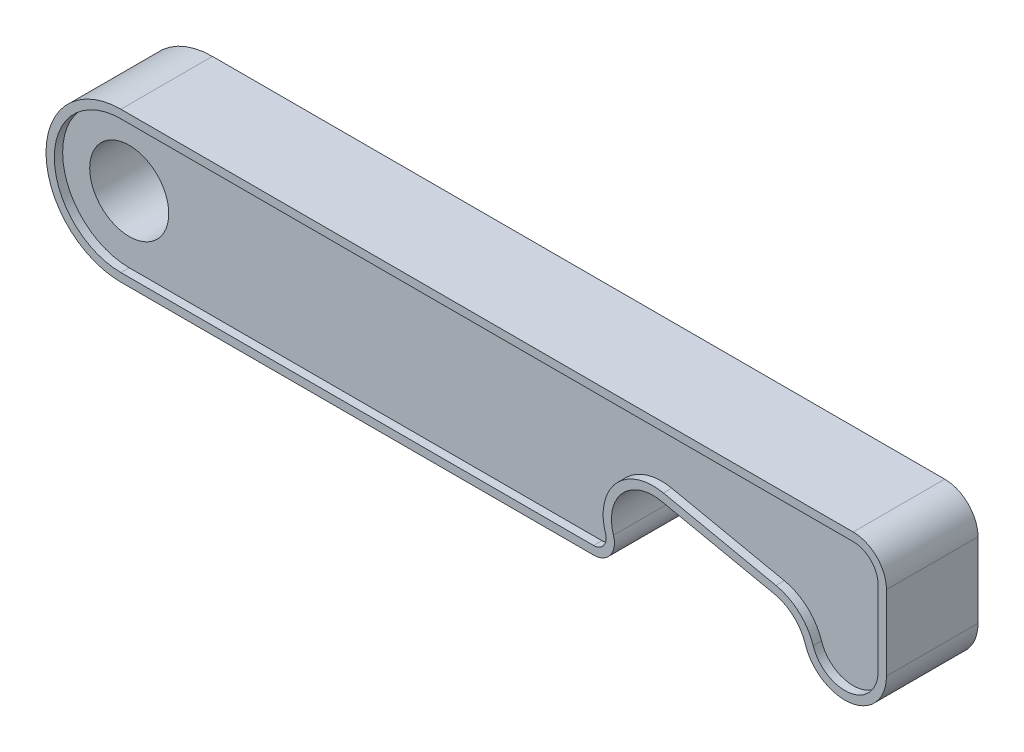
ISO-10303-21;
HEADER;
FILE_DESCRIPTION(('STEP AP214'),'2;1');
FILE_NAME('part.step','',(''),(''),'','','');
FILE_SCHEMA(('AUTOMOTIVE_DESIGN { 1 0 10303 214 1 1 1 1 }'));
ENDSEC;
DATA;
#1=APPLICATION_CONTEXT('core data for automotive mechanical design processes');
#2=APPLICATION_PROTOCOL_DEFINITION('international standard','automotive_design',2000,#1);
#3=PRODUCT_CONTEXT('',#1,'mechanical');
#4=PRODUCT('Part','Part','',(#3));
#5=PRODUCT_RELATED_PRODUCT_CATEGORY('part','',(#4));
#6=PRODUCT_DEFINITION_FORMATION('','',#4);
#7=PRODUCT_DEFINITION_CONTEXT('part definition',#1,'design');
#8=PRODUCT_DEFINITION('design','',#6,#7);
#9=PRODUCT_DEFINITION_SHAPE('','',#8);
#10=(LENGTH_UNIT() NAMED_UNIT(*) SI_UNIT(.MILLI.,.METRE.));
#11=(NAMED_UNIT(*) PLANE_ANGLE_UNIT() SI_UNIT($,.RADIAN.));
#12=(NAMED_UNIT(*) SI_UNIT($,.STERADIAN.) SOLID_ANGLE_UNIT());
#13=UNCERTAINTY_MEASURE_WITH_UNIT(LENGTH_MEASURE(1.E-05),#10,'distance_accuracy_value','');
#14=(GEOMETRIC_REPRESENTATION_CONTEXT(3) GLOBAL_UNCERTAINTY_ASSIGNED_CONTEXT((#13)) GLOBAL_UNIT_ASSIGNED_CONTEXT((#10,
#11,#12)) REPRESENTATION_CONTEXT('',''));
#15=CARTESIAN_POINT('',(0.,0.,0.));
#16=DIRECTION('',(0.,0.,1.));
#17=DIRECTION('',(1.,0.,0.));
#18=AXIS2_PLACEMENT_3D('',#15,#16,#17);
#19=CARTESIAN_POINT('',(56.809405856909,-6.5,4.5));
#20=DIRECTION('',(0.,0.,-1.));
#21=DIRECTION('',(-1.,0.,0.));
#22=AXIS2_PLACEMENT_3D('',#19,#20,#21);
#23=CYLINDRICAL_SURFACE('',#22,2.5);
#24=DIRECTION('',(0.,0.,-1.));
#25=VECTOR('',#24,1.);
#26=CARTESIAN_POINT('',(56.809405856909,-9.,4.5));
#27=LINE('',#26,#25);
#28=CARTESIAN_POINT('',(56.809405856909,-9.,5.5));
#29=VERTEX_POINT('',#28);
#30=CARTESIAN_POINT('',(56.809405856909,-9.,-5.5));
#31=VERTEX_POINT('',#30);
#32=EDGE_CURVE('E469',#29,#31,#27,.T.);
#33=ORIENTED_EDGE('',*,*,#32,.T.);
#34=CARTESIAN_POINT('',(56.809405856909,-6.5,-5.5));
#35=DIRECTION('',(0.,0.,1.));
#36=DIRECTION('',(1.,0.,0.));
#37=AXIS2_PLACEMENT_3D('',#34,#35,#36);
#38=CIRCLE('',#37,2.5);
#39=CARTESIAN_POINT('',(59.1903107477395,-5.73757498675653,-5.5));
#40=VERTEX_POINT('',#39);
#41=EDGE_CURVE('E249',#31,#40,#38,.T.);
#42=ORIENTED_EDGE('',*,*,#41,.T.);
#43=DIRECTION('',(0.,0.,-1.));
#44=VECTOR('',#43,1.);
#45=CARTESIAN_POINT('',(59.1903107477395,-5.73757498675653,4.5));
#46=LINE('',#45,#44);
#47=CARTESIAN_POINT('',(59.1903107477395,-5.73757498675653,5.5));
#48=VERTEX_POINT('',#47);
#49=EDGE_CURVE('E11',#48,#40,#46,.T.);
#50=ORIENTED_EDGE('',*,*,#49,.F.);
#51=CARTESIAN_POINT('',(56.809405856909,-6.5,5.5));
#52=DIRECTION('',(0.,0.,1.));
#53=DIRECTION('',(1.,0.,0.));
#54=AXIS2_PLACEMENT_3D('',#51,#52,#53);
#55=CIRCLE('',#54,2.5);
#56=EDGE_CURVE('E440',#29,#48,#55,.T.);
#57=ORIENTED_EDGE('',*,*,#56,.F.);
#58=EDGE_LOOP('',(#33,#42,#50,#57));
#59=FACE_BOUND('',#58,.T.);
#60=ADVANCED_FACE('F50',(#59),#23,.T.);
#61=CARTESIAN_POINT('',(63.9521205294006,-4.2127249602696,4.5));
#62=DIRECTION('',(0.,0.,-1.));
#63=DIRECTION('',(-1.,0.,0.));
#64=AXIS2_PLACEMENT_3D('',#61,#62,#63);
#65=CYLINDRICAL_SURFACE('',#64,5.00000000000001);
#66=ORIENTED_EDGE('',*,*,#49,.T.);
#67=CARTESIAN_POINT('',(63.9521205294006,-4.2127249602696,-5.5));
#68=DIRECTION('',(0.,0.,-1.));
#69=DIRECTION('',(1.,0.,0.));
#70=AXIS2_PLACEMENT_3D('',#67,#68,#69);
#71=CIRCLE('',#70,5.);
#72=CARTESIAN_POINT('',(64.9855195067217,0.679318227772782,-5.5));
#73=VERTEX_POINT('',#72);
#74=EDGE_CURVE('E361',#40,#73,#71,.T.);
#75=ORIENTED_EDGE('',*,*,#74,.T.);
#76=DIRECTION('',(0.,0.,-1.));
#77=VECTOR('',#76,1.);
#78=CARTESIAN_POINT('',(64.9855195067217,0.679318227772783,4.5));
#79=LINE('',#78,#77);
#80=CARTESIAN_POINT('',(64.9855195067217,0.679318227772782,5.5));
#81=VERTEX_POINT('',#80);
#82=EDGE_CURVE('E53',#81,#73,#79,.T.);
#83=ORIENTED_EDGE('',*,*,#82,.F.);
#84=CARTESIAN_POINT('',(63.9521205294006,-4.2127249602696,5.5));
#85=DIRECTION('',(0.,0.,-1.));
#86=DIRECTION('',(1.,0.,0.));
#87=AXIS2_PLACEMENT_3D('',#84,#85,#86);
#88=CIRCLE('',#87,5.);
#89=EDGE_CURVE('E439',#48,#81,#88,.T.);
#90=ORIENTED_EDGE('',*,*,#89,.F.);
#91=EDGE_LOOP('',(#66,#75,#83,#90));
#92=FACE_BOUND('',#91,.T.);
#93=ADVANCED_FACE('F495',(#92),#65,.F.);
#94=CARTESIAN_POINT('',(2.91332629980599,13.7914962103574,4.5));
#95=DIRECTION('',(0.206679795464213,0.978408637608475,0.));
#96=DIRECTION('',(-0.978408637608475,0.206679795464213,0.));
#97=AXIS2_PLACEMENT_3D('',#94,#95,#96);
#98=PLANE('',#97);
#99=ORIENTED_EDGE('',*,*,#82,.T.);
#100=DIRECTION('',(0.978408637608475,-0.206679795464213,0.));
#101=VECTOR('',#100,1.);
#102=CARTESIAN_POINT('',(64.9855195067217,0.679318227772782,-5.5));
#103=LINE('',#102,#101);
#104=CARTESIAN_POINT('',(78.5166425479577,-2.17900664290652,-5.5));
#105=VERTEX_POINT('',#104);
#106=EDGE_CURVE('E356',#73,#105,#103,.T.);
#107=ORIENTED_EDGE('',*,*,#106,.T.);
#108=DIRECTION('',(0.,0.,-1.));
#109=VECTOR('',#108,1.);
#110=CARTESIAN_POINT('',(78.5166425479577,-2.17900664290653,4.5));
#111=LINE('',#110,#109);
#112=CARTESIAN_POINT('',(78.5166425479577,-2.17900664290652,5.5));
#113=VERTEX_POINT('',#112);
#114=EDGE_CURVE('E481',#113,#105,#111,.T.);
#115=ORIENTED_EDGE('',*,*,#114,.F.);
#116=DIRECTION('',(0.978408637608475,-0.206679795464213,0.));
#117=VECTOR('',#116,1.);
#118=CARTESIAN_POINT('',(64.9855195067217,0.679318227772782,5.5));
#119=LINE('',#118,#117);
#120=EDGE_CURVE('E444',#81,#113,#119,.T.);
#121=ORIENTED_EDGE('',*,*,#120,.F.);
#122=EDGE_LOOP('',(#99,#107,#115,#121));
#123=FACE_BOUND('',#122,.T.);
#124=ADVANCED_FACE('F484',(#123),#98,.F.);
#125=CARTESIAN_POINT('',(77.4832435706367,-7.07104983094887,4.5));
#126=DIRECTION('',(0.,0.,-1.));
#127=DIRECTION('',(-1.,0.,0.));
#128=AXIS2_PLACEMENT_3D('',#125,#126,#127);
#129=CYLINDRICAL_SURFACE('',#128,4.99999999999999);
#130=ORIENTED_EDGE('',*,*,#114,.T.);
#131=CARTESIAN_POINT('',(77.4832435706367,-7.07104983094887,-5.5));
#132=DIRECTION('',(0.,0.,-1.));
#133=DIRECTION('',(1.,0.,0.));
#134=AXIS2_PLACEMENT_3D('',#131,#132,#133);
#135=CIRCLE('',#134,4.99999999999998);
#136=CARTESIAN_POINT('',(82.2416217853183,-5.53552491547443,-5.5));
#137=VERTEX_POINT('',#136);
#138=EDGE_CURVE('E359',#105,#137,#135,.T.);
#139=ORIENTED_EDGE('',*,*,#138,.T.);
#140=DIRECTION('',(0.,0.,-1.));
#141=VECTOR('',#140,1.);
#142=CARTESIAN_POINT('',(82.2416217853183,-5.53552491547443,4.5));
#143=LINE('',#142,#141);
#144=CARTESIAN_POINT('',(82.2416217853183,-5.53552491547443,5.5));
#145=VERTEX_POINT('',#144);
#146=EDGE_CURVE('E479',#145,#137,#143,.T.);
#147=ORIENTED_EDGE('',*,*,#146,.F.);
#148=CARTESIAN_POINT('',(77.4832435706367,-7.07104983094887,5.5));
#149=DIRECTION('',(0.,0.,-1.));
#150=DIRECTION('',(1.,0.,0.));
#151=AXIS2_PLACEMENT_3D('',#148,#149,#150);
#152=CIRCLE('',#151,4.99999999999998);
#153=EDGE_CURVE('E446',#113,#145,#152,.T.);
#154=ORIENTED_EDGE('',*,*,#153,.F.);
#155=EDGE_LOOP('',(#130,#139,#147,#154));
#156=FACE_BOUND('',#155,.T.);
#157=ADVANCED_FACE('F522',(#156),#129,.F.);
#158=CARTESIAN_POINT('',(87.,-4.,4.5));
#159=DIRECTION('',(0.,0.,-1.));
#160=DIRECTION('',(-1.,0.,0.));
#161=AXIS2_PLACEMENT_3D('',#158,#159,#160);
#162=CYLINDRICAL_SURFACE('',#161,4.99999999999999);
#163=ORIENTED_EDGE('',*,*,#146,.T.);
#164=CARTESIAN_POINT('',(87.,-4.,-5.5));
#165=DIRECTION('',(0.,0.,1.));
#166=DIRECTION('',(1.,0.,0.));
#167=AXIS2_PLACEMENT_3D('',#164,#165,#166);
#168=CIRCLE('',#167,5.);
#169=CARTESIAN_POINT('',(92.,-4.,-5.5));
#170=VERTEX_POINT('',#169);
#171=EDGE_CURVE('E353',#137,#170,#168,.T.);
#172=ORIENTED_EDGE('',*,*,#171,.T.);
#173=DIRECTION('',(0.,0.,-1.));
#174=VECTOR('',#173,1.);
#175=CARTESIAN_POINT('',(92.,-4.,4.5));
#176=LINE('',#175,#174);
#177=CARTESIAN_POINT('',(92.,-4.,5.5));
#178=VERTEX_POINT('',#177);
#179=EDGE_CURVE('E480',#178,#170,#176,.T.);
#180=ORIENTED_EDGE('',*,*,#179,.F.);
#181=CARTESIAN_POINT('',(87.,-4.,5.5));
#182=DIRECTION('',(0.,0.,1.));
#183=DIRECTION('',(1.,0.,0.));
#184=AXIS2_PLACEMENT_3D('',#181,#182,#183);
#185=CIRCLE('',#184,5.);
#186=EDGE_CURVE('E448',#145,#178,#185,.T.);
#187=ORIENTED_EDGE('',*,*,#186,.F.);
#188=EDGE_LOOP('',(#163,#172,#180,#187));
#189=FACE_BOUND('',#188,.T.);
#190=ADVANCED_FACE('F523',(#189),#162,.T.);
#191=CARTESIAN_POINT('',(92.,-1.41861830924326E-13,4.5));
#192=DIRECTION('',(1.,0.,0.));
#193=DIRECTION('',(0.,1.,0.));
#194=AXIS2_PLACEMENT_3D('',#191,#192,#193);
#195=PLANE('',#194);
#196=ORIENTED_EDGE('',*,*,#179,.T.);
#197=DIRECTION('',(0.,1.,0.));
#198=VECTOR('',#197,1.);
#199=CARTESIAN_POINT('',(92.,-4.,-5.5));
#200=LINE('',#199,#198);
#201=CARTESIAN_POINT('',(92.,5.,-5.5));
#202=VERTEX_POINT('',#201);
#203=EDGE_CURVE('E351',#170,#202,#200,.T.);
#204=ORIENTED_EDGE('',*,*,#203,.T.);
#205=DIRECTION('',(0.,0.,-1.));
#206=VECTOR('',#205,1.);
#207=CARTESIAN_POINT('',(92.,5.,4.5));
#208=LINE('',#207,#206);
#209=CARTESIAN_POINT('',(92.,5.,5.5));
#210=VERTEX_POINT('',#209);
#211=EDGE_CURVE('E474',#210,#202,#208,.T.);
#212=ORIENTED_EDGE('',*,*,#211,.F.);
#213=DIRECTION('',(0.,1.,0.));
#214=VECTOR('',#213,1.);
#215=CARTESIAN_POINT('',(92.,-4.,5.5));
#216=LINE('',#215,#214);
#217=EDGE_CURVE('E454',#178,#210,#216,.T.);
#218=ORIENTED_EDGE('',*,*,#217,.F.);
#219=EDGE_LOOP('',(#196,#204,#212,#218));
#220=FACE_BOUND('',#219,.T.);
#221=ADVANCED_FACE('F517',(#220),#195,.T.);
#222=CARTESIAN_POINT('',(88.,5.,4.5));
#223=DIRECTION('',(0.,0.,-1.));
#224=DIRECTION('',(-1.,0.,0.));
#225=AXIS2_PLACEMENT_3D('',#222,#223,#224);
#226=CYLINDRICAL_SURFACE('',#225,4.);
#227=ORIENTED_EDGE('',*,*,#211,.T.);
#228=CARTESIAN_POINT('',(88.,5.,-5.5));
#229=DIRECTION('',(0.,0.,1.));
#230=DIRECTION('',(1.,0.,0.));
#231=AXIS2_PLACEMENT_3D('',#228,#229,#230);
#232=CIRCLE('',#231,4.);
#233=CARTESIAN_POINT('',(88.,9.,-5.5));
#234=VERTEX_POINT('',#233);
#235=EDGE_CURVE('E346',#202,#234,#232,.T.);
#236=ORIENTED_EDGE('',*,*,#235,.T.);
#237=DIRECTION('',(0.,0.,-1.));
#238=VECTOR('',#237,1.);
#239=CARTESIAN_POINT('',(88.,9.,4.5));
#240=LINE('',#239,#238);
#241=CARTESIAN_POINT('',(88.,9.,5.5));
#242=VERTEX_POINT('',#241);
#243=EDGE_CURVE('E471',#242,#234,#240,.T.);
#244=ORIENTED_EDGE('',*,*,#243,.F.);
#245=CARTESIAN_POINT('',(88.,5.,5.5));
#246=DIRECTION('',(0.,0.,1.));
#247=DIRECTION('',(1.,0.,0.));
#248=AXIS2_PLACEMENT_3D('',#245,#246,#247);
#249=CIRCLE('',#248,4.);
#250=EDGE_CURVE('E451',#210,#242,#249,.T.);
#251=ORIENTED_EDGE('',*,*,#250,.F.);
#252=EDGE_LOOP('',(#227,#236,#244,#251));
#253=FACE_BOUND('',#252,.T.);
#254=ADVANCED_FACE('F514',(#253),#226,.T.);
#255=CARTESIAN_POINT('',(0.,9.,4.5));
#256=DIRECTION('',(0.,1.,0.));
#257=DIRECTION('',(0.,0.,1.));
#258=AXIS2_PLACEMENT_3D('',#255,#256,#257);
#259=PLANE('',#258);
#260=ORIENTED_EDGE('',*,*,#243,.T.);
#261=DIRECTION('',(-1.,0.,0.));
#262=VECTOR('',#261,1.);
#263=CARTESIAN_POINT('',(88.,9.,-5.5));
#264=LINE('',#263,#262);
#265=CARTESIAN_POINT('',(0.,9.,-5.5));
#266=VERTEX_POINT('',#265);
#267=EDGE_CURVE('E341',#234,#266,#264,.T.);
#268=ORIENTED_EDGE('',*,*,#267,.T.);
#269=DIRECTION('',(0.,0.,-1.));
#270=VECTOR('',#269,1.);
#271=CARTESIAN_POINT('',(0.,9.,4.5));
#272=LINE('',#271,#270);
#273=CARTESIAN_POINT('',(0.,9.,5.5));
#274=VERTEX_POINT('',#273);
#275=EDGE_CURVE('E473',#274,#266,#272,.T.);
#276=ORIENTED_EDGE('',*,*,#275,.F.);
#277=DIRECTION('',(-1.,0.,0.));
#278=VECTOR('',#277,1.);
#279=CARTESIAN_POINT('',(88.,9.,5.5));
#280=LINE('',#279,#278);
#281=EDGE_CURVE('E456',#242,#274,#280,.T.);
#282=ORIENTED_EDGE('',*,*,#281,.F.);
#283=EDGE_LOOP('',(#260,#268,#276,#282));
#284=FACE_BOUND('',#283,.T.);
#285=ADVANCED_FACE('F510',(#284),#259,.T.);
#286=CARTESIAN_POINT('',(0.,0.,4.5));
#287=DIRECTION('',(0.,0.,-1.));
#288=DIRECTION('',(-1.,0.,0.));
#289=AXIS2_PLACEMENT_3D('',#286,#287,#288);
#290=CYLINDRICAL_SURFACE('',#289,9.);
#291=ORIENTED_EDGE('',*,*,#275,.T.);
#292=CARTESIAN_POINT('',(0.,0.,-5.5));
#293=DIRECTION('',(0.,0.,1.));
#294=DIRECTION('',(1.,0.,0.));
#295=AXIS2_PLACEMENT_3D('',#292,#293,#294);
#296=CIRCLE('',#295,9.);
#297=CARTESIAN_POINT('',(0.,-9.,-5.5));
#298=VERTEX_POINT('',#297);
#299=EDGE_CURVE('E344',#266,#298,#296,.T.);
#300=ORIENTED_EDGE('',*,*,#299,.T.);
#301=DIRECTION('',(0.,0.,-1.));
#302=VECTOR('',#301,1.);
#303=CARTESIAN_POINT('',(0.,-9.,4.5));
#304=LINE('',#303,#302);
#305=CARTESIAN_POINT('',(0.,-9.,5.5));
#306=VERTEX_POINT('',#305);
#307=EDGE_CURVE('E470',#306,#298,#304,.T.);
#308=ORIENTED_EDGE('',*,*,#307,.F.);
#309=CARTESIAN_POINT('',(0.,0.,5.5));
#310=DIRECTION('',(0.,0.,1.));
#311=DIRECTION('',(1.,0.,0.));
#312=AXIS2_PLACEMENT_3D('',#309,#310,#311);
#313=CIRCLE('',#312,9.);
#314=EDGE_CURVE('E461',#274,#306,#313,.T.);
#315=ORIENTED_EDGE('',*,*,#314,.F.);
#316=EDGE_LOOP('',(#291,#300,#308,#315));
#317=FACE_BOUND('',#316,.T.);
#318=ADVANCED_FACE('F502',(#317),#290,.T.);
#319=CARTESIAN_POINT('',(0.,-9.,4.5));
#320=DIRECTION('',(0.,1.,0.));
#321=DIRECTION('',(-1.,0.,0.));
#322=AXIS2_PLACEMENT_3D('',#319,#320,#321);
#323=PLANE('',#322);
#324=ORIENTED_EDGE('',*,*,#307,.T.);
#325=DIRECTION('',(1.,0.,0.));
#326=VECTOR('',#325,1.);
#327=CARTESIAN_POINT('',(0.,-9.,-5.5));
#328=LINE('',#327,#326);
#329=EDGE_CURVE('E338',#298,#31,#328,.T.);
#330=ORIENTED_EDGE('',*,*,#329,.T.);
#331=ORIENTED_EDGE('',*,*,#32,.F.);
#332=DIRECTION('',(1.,0.,0.));
#333=VECTOR('',#332,1.);
#334=CARTESIAN_POINT('',(0.,-9.,5.5));
#335=LINE('',#334,#333);
#336=EDGE_CURVE('E463',#306,#29,#335,.T.);
#337=ORIENTED_EDGE('',*,*,#336,.F.);
#338=EDGE_LOOP('',(#324,#330,#331,#337));
#339=FACE_BOUND('',#338,.T.);
#340=ADVANCED_FACE('F499',(#339),#323,.F.);
#341=CARTESIAN_POINT('',(56.809405856909,-6.5,5.5));
#342=DIRECTION('',(0.,0.,1.));
#343=DIRECTION('',(1.,0.,0.));
#344=AXIS2_PLACEMENT_3D('',#341,#342,#343);
#345=PLANE('',#344);
#346=ORIENTED_EDGE('',*,*,#56,.T.);
#347=ORIENTED_EDGE('',*,*,#89,.T.);
#348=ORIENTED_EDGE('',*,*,#120,.T.);
#349=ORIENTED_EDGE('',*,*,#153,.T.);
#350=ORIENTED_EDGE('',*,*,#186,.T.);
#351=ORIENTED_EDGE('',*,*,#217,.T.);
#352=ORIENTED_EDGE('',*,*,#250,.T.);
#353=ORIENTED_EDGE('',*,*,#281,.T.);
#354=ORIENTED_EDGE('',*,*,#314,.T.);
#355=ORIENTED_EDGE('',*,*,#336,.T.);
#356=EDGE_LOOP('',(#346,#347,#348,#349,#350,#351,#352,#353,#354,#355));
#357=FACE_BOUND('',#356,.T.);
#358=DIRECTION('',(0.978408637608475,-0.206679795464213,0.));
#359=VECTOR('',#358,1.);
#360=CARTESIAN_POINT('',(65.1921993021859,1.65772686538126,5.5));
#361=LINE('',#360,#359);
#362=CARTESIAN_POINT('',(65.1921993021859,1.65772686538126,5.5));
#363=VERTEX_POINT('',#362);
#364=CARTESIAN_POINT('',(78.7233223434219,-1.20059800529805,5.5));
#365=VERTEX_POINT('',#364);
#366=EDGE_CURVE('E369',#363,#365,#361,.T.);
#367=ORIENTED_EDGE('',*,*,#366,.F.);
#368=CARTESIAN_POINT('',(63.9521205294006,-4.2127249602696,5.5));
#369=DIRECTION('',(0.,0.,-1.));
#370=DIRECTION('',(1.,0.,0.));
#371=AXIS2_PLACEMENT_3D('',#368,#369,#370);
#372=CIRCLE('',#371,6.);
#373=CARTESIAN_POINT('',(58.2379487914073,-6.04254499205392,5.5));
#374=VERTEX_POINT('',#373);
#375=EDGE_CURVE('E370',#374,#363,#372,.T.);
#376=ORIENTED_EDGE('',*,*,#375,.F.);
#377=CARTESIAN_POINT('',(56.809405856909,-6.5,5.5));
#378=DIRECTION('',(0.,0.,1.));
#379=DIRECTION('',(1.,0.,0.));
#380=AXIS2_PLACEMENT_3D('',#377,#378,#379);
#381=CIRCLE('',#380,1.5);
#382=CARTESIAN_POINT('',(56.809405856909,-8.,5.5));
#383=VERTEX_POINT('',#382);
#384=EDGE_CURVE('E390',#383,#374,#381,.T.);
#385=ORIENTED_EDGE('',*,*,#384,.F.);
#386=DIRECTION('',(1.,0.,0.));
#387=VECTOR('',#386,1.);
#388=CARTESIAN_POINT('',(0.,-8.,5.5));
#389=LINE('',#388,#387);
#390=CARTESIAN_POINT('',(0.,-8.,5.5));
#391=VERTEX_POINT('',#390);
#392=EDGE_CURVE('E383',#391,#383,#389,.T.);
#393=ORIENTED_EDGE('',*,*,#392,.F.);
#394=CARTESIAN_POINT('',(0.,0.,5.5));
#395=DIRECTION('',(0.,0.,1.));
#396=DIRECTION('',(1.,0.,0.));
#397=AXIS2_PLACEMENT_3D('',#394,#395,#396);
#398=CIRCLE('',#397,8.);
#399=CARTESIAN_POINT('',(0.,8.,5.5));
#400=VERTEX_POINT('',#399);
#401=EDGE_CURVE('E385',#400,#391,#398,.T.);
#402=ORIENTED_EDGE('',*,*,#401,.F.);
#403=DIRECTION('',(-1.,0.,0.));
#404=VECTOR('',#403,1.);
#405=CARTESIAN_POINT('',(88.,8.,5.5));
#406=LINE('',#405,#404);
#407=CARTESIAN_POINT('',(88.,7.99999999999999,5.5));
#408=VERTEX_POINT('',#407);
#409=EDGE_CURVE('E379',#408,#400,#406,.T.);
#410=ORIENTED_EDGE('',*,*,#409,.F.);
#411=CARTESIAN_POINT('',(88.,5.,5.5));
#412=DIRECTION('',(0.,0.,1.));
#413=DIRECTION('',(1.,0.,0.));
#414=AXIS2_PLACEMENT_3D('',#411,#412,#413);
#415=CIRCLE('',#414,3.);
#416=CARTESIAN_POINT('',(91.,5.,5.5));
#417=VERTEX_POINT('',#416);
#418=EDGE_CURVE('E378',#417,#408,#415,.T.);
#419=ORIENTED_EDGE('',*,*,#418,.F.);
#420=DIRECTION('',(0.,1.,0.));
#421=VECTOR('',#420,1.);
#422=CARTESIAN_POINT('',(91.,-4.,5.5));
#423=LINE('',#422,#421);
#424=CARTESIAN_POINT('',(91.,-4.,5.5));
#425=VERTEX_POINT('',#424);
#426=EDGE_CURVE('E376',#425,#417,#423,.T.);
#427=ORIENTED_EDGE('',*,*,#426,.F.);
#428=CARTESIAN_POINT('',(87.,-4.,5.5));
#429=DIRECTION('',(0.,0.,1.));
#430=DIRECTION('',(1.,0.,0.));
#431=AXIS2_PLACEMENT_3D('',#428,#429,#430);
#432=CIRCLE('',#431,3.99999999999999);
#433=CARTESIAN_POINT('',(83.1932974282547,-5.22841993237955,5.5));
#434=VERTEX_POINT('',#433);
#435=EDGE_CURVE('E372',#434,#425,#432,.T.);
#436=ORIENTED_EDGE('',*,*,#435,.F.);
#437=CARTESIAN_POINT('',(77.4832435706367,-7.07104983094887,5.5));
#438=DIRECTION('',(0.,0.,-1.));
#439=DIRECTION('',(1.,0.,0.));
#440=AXIS2_PLACEMENT_3D('',#437,#438,#439);
#441=CIRCLE('',#440,5.99999999999998);
#442=EDGE_CURVE('E375',#365,#434,#441,.T.);
#443=ORIENTED_EDGE('',*,*,#442,.F.);
#444=EDGE_LOOP('',(#367,#376,#385,#393,#402,#410,#419,#427,#436,#443));
#445=FACE_BOUND('',#444,.T.);
#446=ADVANCED_FACE('F503',(#357,#445),#345,.T.);
#447=CARTESIAN_POINT('',(63.9521205294006,-4.2127249602696,5.5));
#448=DIRECTION('',(0.,0.,-1.));
#449=DIRECTION('',(-1.,0.,0.));
#450=AXIS2_PLACEMENT_3D('',#447,#448,#449);
#451=CYLINDRICAL_SURFACE('',#450,6.);
#452=CARTESIAN_POINT('',(63.9521205294006,-4.2127249602696,4.5));
#453=DIRECTION('',(0.,0.,-1.));
#454=DIRECTION('',(1.,0.,0.));
#455=AXIS2_PLACEMENT_3D('',#452,#453,#454);
#456=CIRCLE('',#455,6.);
#457=CARTESIAN_POINT('',(58.2379487914073,-6.04254499205392,4.5));
#458=VERTEX_POINT('',#457);
#459=CARTESIAN_POINT('',(65.1921993021859,1.65772686538126,4.5));
#460=VERTEX_POINT('',#459);
#461=EDGE_CURVE('E368',#458,#460,#456,.T.);
#462=ORIENTED_EDGE('',*,*,#461,.F.);
#463=DIRECTION('',(0.,0.,-1.));
#464=VECTOR('',#463,1.);
#465=CARTESIAN_POINT('',(58.2379487914073,-6.04254499205392,5.5));
#466=LINE('',#465,#464);
#467=EDGE_CURVE('E386',#374,#458,#466,.T.);
#468=ORIENTED_EDGE('',*,*,#467,.F.);
#469=ORIENTED_EDGE('',*,*,#375,.T.);
#470=DIRECTION('',(0.,0.,-1.));
#471=VECTOR('',#470,1.);
#472=CARTESIAN_POINT('',(65.1921993021859,1.65772686538126,5.5));
#473=LINE('',#472,#471);
#474=EDGE_CURVE('E432',#363,#460,#473,.T.);
#475=ORIENTED_EDGE('',*,*,#474,.T.);
#476=EDGE_LOOP('',(#462,#468,#469,#475));
#477=FACE_BOUND('',#476,.T.);
#478=ADVANCED_FACE('F761',(#477),#451,.T.);
#479=CARTESIAN_POINT('',(65.1921993021859,1.65772686538126,5.5));
#480=DIRECTION('',(0.206679795464213,0.978408637608475,0.));
#481=DIRECTION('',(-0.978408637608475,0.206679795464213,0.));
#482=AXIS2_PLACEMENT_3D('',#479,#480,#481);
#483=PLANE('',#482);
#484=DIRECTION('',(0.978408637608475,-0.206679795464213,0.));
#485=VECTOR('',#484,1.);
#486=CARTESIAN_POINT('',(65.1921993021859,1.65772686538126,4.5));
#487=LINE('',#486,#485);
#488=CARTESIAN_POINT('',(78.7233223434219,-1.20059800529804,4.5));
#489=VERTEX_POINT('',#488);
#490=EDGE_CURVE('E391',#460,#489,#487,.T.);
#491=ORIENTED_EDGE('',*,*,#490,.F.);
#492=ORIENTED_EDGE('',*,*,#474,.F.);
#493=ORIENTED_EDGE('',*,*,#366,.T.);
#494=DIRECTION('',(0.,0.,-1.));
#495=VECTOR('',#494,1.);
#496=CARTESIAN_POINT('',(78.7233223434219,-1.20059800529805,5.5));
#497=LINE('',#496,#495);
#498=EDGE_CURVE('E431',#365,#489,#497,.T.);
#499=ORIENTED_EDGE('',*,*,#498,.T.);
#500=EDGE_LOOP('',(#491,#492,#493,#499));
#501=FACE_BOUND('',#500,.T.);
#502=ADVANCED_FACE('F768',(#501),#483,.T.);
#503=CARTESIAN_POINT('',(77.4832435706367,-7.07104983094887,5.5));
#504=DIRECTION('',(0.,0.,-1.));
#505=DIRECTION('',(-1.,0.,0.));
#506=AXIS2_PLACEMENT_3D('',#503,#504,#505);
#507=CYLINDRICAL_SURFACE('',#506,5.99999999999998);
#508=CARTESIAN_POINT('',(77.4832435706367,-7.07104983094887,4.5));
#509=DIRECTION('',(0.,0.,-1.));
#510=DIRECTION('',(1.,0.,0.));
#511=AXIS2_PLACEMENT_3D('',#508,#509,#510);
#512=CIRCLE('',#511,5.99999999999998);
#513=CARTESIAN_POINT('',(83.1932974282547,-5.22841993237955,4.5));
#514=VERTEX_POINT('',#513);
#515=EDGE_CURVE('E394',#489,#514,#512,.T.);
#516=ORIENTED_EDGE('',*,*,#515,.F.);
#517=ORIENTED_EDGE('',*,*,#498,.F.);
#518=ORIENTED_EDGE('',*,*,#442,.T.);
#519=DIRECTION('',(0.,0.,-1.));
#520=VECTOR('',#519,1.);
#521=CARTESIAN_POINT('',(83.1932974282547,-5.22841993237955,5.5));
#522=LINE('',#521,#520);
#523=EDGE_CURVE('E428',#434,#514,#522,.T.);
#524=ORIENTED_EDGE('',*,*,#523,.T.);
#525=EDGE_LOOP('',(#516,#517,#518,#524));
#526=FACE_BOUND('',#525,.T.);
#527=ADVANCED_FACE('F779',(#526),#507,.T.);
#528=CARTESIAN_POINT('',(87.,-4.,5.5));
#529=DIRECTION('',(0.,0.,-1.));
#530=DIRECTION('',(-1.,0.,0.));
#531=AXIS2_PLACEMENT_3D('',#528,#529,#530);
#532=CYLINDRICAL_SURFACE('',#531,3.99999999999999);
#533=CARTESIAN_POINT('',(87.,-4.,4.5));
#534=DIRECTION('',(0.,0.,1.));
#535=DIRECTION('',(1.,0.,0.));
#536=AXIS2_PLACEMENT_3D('',#533,#534,#535);
#537=CIRCLE('',#536,3.99999999999999);
#538=CARTESIAN_POINT('',(91.,-4.,4.5));
#539=VERTEX_POINT('',#538);
#540=EDGE_CURVE('E395',#514,#539,#537,.T.);
#541=ORIENTED_EDGE('',*,*,#540,.F.);
#542=ORIENTED_EDGE('',*,*,#523,.F.);
#543=ORIENTED_EDGE('',*,*,#435,.T.);
#544=DIRECTION('',(0.,0.,-1.));
#545=VECTOR('',#544,1.);
#546=CARTESIAN_POINT('',(91.,-4.,5.5));
#547=LINE('',#546,#545);
#548=EDGE_CURVE('E422',#425,#539,#547,.T.);
#549=ORIENTED_EDGE('',*,*,#548,.T.);
#550=EDGE_LOOP('',(#541,#542,#543,#549));
#551=FACE_BOUND('',#550,.T.);
#552=ADVANCED_FACE('F790',(#551),#532,.F.);
#553=CARTESIAN_POINT('',(91.,-4.,5.5));
#554=DIRECTION('',(-1.,0.,0.));
#555=DIRECTION('',(0.,0.,1.));
#556=AXIS2_PLACEMENT_3D('',#553,#554,#555);
#557=PLANE('',#556);
#558=DIRECTION('',(0.,1.,0.));
#559=VECTOR('',#558,1.);
#560=CARTESIAN_POINT('',(91.,-4.,4.5));
#561=LINE('',#560,#559);
#562=CARTESIAN_POINT('',(91.,5.,4.5));
#563=VERTEX_POINT('',#562);
#564=EDGE_CURVE('E399',#539,#563,#561,.T.);
#565=ORIENTED_EDGE('',*,*,#564,.F.);
#566=ORIENTED_EDGE('',*,*,#548,.F.);
#567=ORIENTED_EDGE('',*,*,#426,.T.);
#568=DIRECTION('',(0.,0.,-1.));
#569=VECTOR('',#568,1.);
#570=CARTESIAN_POINT('',(91.,5.,5.5));
#571=LINE('',#570,#569);
#572=EDGE_CURVE('E425',#417,#563,#571,.T.);
#573=ORIENTED_EDGE('',*,*,#572,.T.);
#574=EDGE_LOOP('',(#565,#566,#567,#573));
#575=FACE_BOUND('',#574,.T.);
#576=ADVANCED_FACE('F798',(#575),#557,.T.);
#577=CARTESIAN_POINT('',(88.,5.,5.5));
#578=DIRECTION('',(0.,0.,-1.));
#579=DIRECTION('',(-1.,0.,0.));
#580=AXIS2_PLACEMENT_3D('',#577,#578,#579);
#581=CYLINDRICAL_SURFACE('',#580,3.);
#582=CARTESIAN_POINT('',(88.,5.,4.5));
#583=DIRECTION('',(0.,0.,1.));
#584=DIRECTION('',(1.,0.,0.));
#585=AXIS2_PLACEMENT_3D('',#582,#583,#584);
#586=CIRCLE('',#585,3.);
#587=CARTESIAN_POINT('',(88.,8.,4.5));
#588=VERTEX_POINT('',#587);
#589=EDGE_CURVE('E400',#563,#588,#586,.T.);
#590=ORIENTED_EDGE('',*,*,#589,.F.);
#591=ORIENTED_EDGE('',*,*,#572,.F.);
#592=ORIENTED_EDGE('',*,*,#418,.T.);
#593=DIRECTION('',(0.,0.,-1.));
#594=VECTOR('',#593,1.);
#595=CARTESIAN_POINT('',(88.,7.99999999999999,5.5));
#596=LINE('',#595,#594);
#597=EDGE_CURVE('E420',#408,#588,#596,.T.);
#598=ORIENTED_EDGE('',*,*,#597,.T.);
#599=EDGE_LOOP('',(#590,#591,#592,#598));
#600=FACE_BOUND('',#599,.T.);
#601=ADVANCED_FACE('F804',(#600),#581,.F.);
#602=CARTESIAN_POINT('',(88.,8.,5.5));
#603=DIRECTION('',(0.,-1.,0.));
#604=DIRECTION('',(1.,0.,0.));
#605=AXIS2_PLACEMENT_3D('',#602,#603,#604);
#606=PLANE('',#605);
#607=DIRECTION('',(-1.,0.,0.));
#608=VECTOR('',#607,1.);
#609=CARTESIAN_POINT('',(88.,8.,4.5));
#610=LINE('',#609,#608);
#611=CARTESIAN_POINT('',(0.,8.,4.5));
#612=VERTEX_POINT('',#611);
#613=EDGE_CURVE('E402',#588,#612,#610,.T.);
#614=ORIENTED_EDGE('',*,*,#613,.F.);
#615=ORIENTED_EDGE('',*,*,#597,.F.);
#616=ORIENTED_EDGE('',*,*,#409,.T.);
#617=DIRECTION('',(0.,0.,-1.));
#618=VECTOR('',#617,1.);
#619=CARTESIAN_POINT('',(0.,8.,5.5));
#620=LINE('',#619,#618);
#621=EDGE_CURVE('E418',#400,#612,#620,.T.);
#622=ORIENTED_EDGE('',*,*,#621,.T.);
#623=EDGE_LOOP('',(#614,#615,#616,#622));
#624=FACE_BOUND('',#623,.T.);
#625=ADVANCED_FACE('F812',(#624),#606,.T.);
#626=CARTESIAN_POINT('',(0.,0.,5.5));
#627=DIRECTION('',(0.,0.,-1.));
#628=DIRECTION('',(-1.,0.,0.));
#629=AXIS2_PLACEMENT_3D('',#626,#627,#628);
#630=CYLINDRICAL_SURFACE('',#629,8.);
#631=CARTESIAN_POINT('',(0.,0.,4.5));
#632=DIRECTION('',(0.,0.,1.));
#633=DIRECTION('',(1.,0.,0.));
#634=AXIS2_PLACEMENT_3D('',#631,#632,#633);
#635=CIRCLE('',#634,8.);
#636=CARTESIAN_POINT('',(0.,-8.,4.5));
#637=VERTEX_POINT('',#636);
#638=EDGE_CURVE('E401',#612,#637,#635,.T.);
#639=ORIENTED_EDGE('',*,*,#638,.F.);
#640=ORIENTED_EDGE('',*,*,#621,.F.);
#641=ORIENTED_EDGE('',*,*,#401,.T.);
#642=DIRECTION('',(0.,0.,-1.));
#643=VECTOR('',#642,1.);
#644=CARTESIAN_POINT('',(0.,-8.,5.5));
#645=LINE('',#644,#643);
#646=EDGE_CURVE('E412',#391,#637,#645,.T.);
#647=ORIENTED_EDGE('',*,*,#646,.T.);
#648=EDGE_LOOP('',(#639,#640,#641,#647));
#649=FACE_BOUND('',#648,.T.);
#650=ADVANCED_FACE('F822',(#649),#630,.F.);
#651=CARTESIAN_POINT('',(0.,-8.,5.5));
#652=DIRECTION('',(0.,1.,0.));
#653=DIRECTION('',(0.,0.,1.));
#654=AXIS2_PLACEMENT_3D('',#651,#652,#653);
#655=PLANE('',#654);
#656=DIRECTION('',(1.,0.,0.));
#657=VECTOR('',#656,1.);
#658=CARTESIAN_POINT('',(0.,-8.,4.5));
#659=LINE('',#658,#657);
#660=CARTESIAN_POINT('',(56.809405856909,-8.,4.5));
#661=VERTEX_POINT('',#660);
#662=EDGE_CURVE('E403',#637,#661,#659,.T.);
#663=ORIENTED_EDGE('',*,*,#662,.F.);
#664=ORIENTED_EDGE('',*,*,#646,.F.);
#665=ORIENTED_EDGE('',*,*,#392,.T.);
#666=DIRECTION('',(0.,0.,-1.));
#667=VECTOR('',#666,1.);
#668=CARTESIAN_POINT('',(56.809405856909,-8.,5.5));
#669=LINE('',#668,#667);
#670=EDGE_CURVE('E410',#383,#661,#669,.T.);
#671=ORIENTED_EDGE('',*,*,#670,.T.);
#672=EDGE_LOOP('',(#663,#664,#665,#671));
#673=FACE_BOUND('',#672,.T.);
#674=ADVANCED_FACE('F832',(#673),#655,.T.);
#675=CARTESIAN_POINT('',(56.809405856909,-6.5,5.5));
#676=DIRECTION('',(0.,0.,-1.));
#677=DIRECTION('',(-1.,0.,0.));
#678=AXIS2_PLACEMENT_3D('',#675,#676,#677);
#679=CYLINDRICAL_SURFACE('',#678,1.5);
#680=CARTESIAN_POINT('',(56.809405856909,-6.5,4.5));
#681=DIRECTION('',(0.,0.,1.));
#682=DIRECTION('',(1.,0.,0.));
#683=AXIS2_PLACEMENT_3D('',#680,#681,#682);
#684=CIRCLE('',#683,1.5);
#685=EDGE_CURVE('E367',#661,#458,#684,.T.);
#686=ORIENTED_EDGE('',*,*,#685,.F.);
#687=ORIENTED_EDGE('',*,*,#670,.F.);
#688=ORIENTED_EDGE('',*,*,#384,.T.);
#689=ORIENTED_EDGE('',*,*,#467,.T.);
#690=EDGE_LOOP('',(#686,#687,#688,#689));
#691=FACE_BOUND('',#690,.T.);
#692=ADVANCED_FACE('F748',(#691),#679,.F.);
#693=CARTESIAN_POINT('',(0.,0.,4.5));
#694=DIRECTION('',(0.,0.,1.));
#695=DIRECTION('',(1.,0.,0.));
#696=AXIS2_PLACEMENT_3D('',#693,#694,#695);
#697=PLANE('',#696);
#698=CARTESIAN_POINT('',(0.,0.,4.5));
#699=DIRECTION('',(0.,0.,1.));
#700=DIRECTION('',(1.,0.,0.));
#701=AXIS2_PLACEMENT_3D('',#698,#699,#700);
#702=CIRCLE('',#701,4.75);
#703=CARTESIAN_POINT('',(4.75,0.,4.5));
#704=VERTEX_POINT('',#703);
#705=EDGE_CURVE('E290',#704,#704,#702,.T.);
#706=ORIENTED_EDGE('',*,*,#705,.F.);
#707=EDGE_LOOP('',(#706));
#708=FACE_BOUND('',#707,.T.);
#709=ORIENTED_EDGE('',*,*,#461,.T.);
#710=ORIENTED_EDGE('',*,*,#490,.T.);
#711=ORIENTED_EDGE('',*,*,#515,.T.);
#712=ORIENTED_EDGE('',*,*,#540,.T.);
#713=ORIENTED_EDGE('',*,*,#564,.T.);
#714=ORIENTED_EDGE('',*,*,#589,.T.);
#715=ORIENTED_EDGE('',*,*,#613,.T.);
#716=ORIENTED_EDGE('',*,*,#638,.T.);
#717=ORIENTED_EDGE('',*,*,#662,.T.);
#718=ORIENTED_EDGE('',*,*,#685,.T.);
#719=EDGE_LOOP('',(#709,#710,#711,#712,#713,#714,#715,#716,#717,#718));
#720=FACE_BOUND('',#719,.T.);
#721=ADVANCED_FACE('F622',(#708,#720),#697,.T.);
#722=CARTESIAN_POINT('',(56.809405856909,-6.5,-5.5));
#723=DIRECTION('',(0.,0.,-1.));
#724=DIRECTION('',(1.,0.,0.));
#725=AXIS2_PLACEMENT_3D('',#722,#723,#724);
#726=PLANE('',#725);
#727=CARTESIAN_POINT('',(63.9521205294006,-4.2127249602696,-5.5));
#728=DIRECTION('',(0.,0.,-1.));
#729=DIRECTION('',(1.,0.,0.));
#730=AXIS2_PLACEMENT_3D('',#727,#728,#729);
#731=CIRCLE('',#730,6.);
#732=CARTESIAN_POINT('',(58.2379487914073,-6.04254499205392,-5.5));
#733=VERTEX_POINT('',#732);
#734=CARTESIAN_POINT('',(65.1921993021859,1.65772686538126,-5.5));
#735=VERTEX_POINT('',#734);
#736=EDGE_CURVE('E253',#733,#735,#731,.T.);
#737=ORIENTED_EDGE('',*,*,#736,.T.);
#738=DIRECTION('',(0.978408637608475,-0.206679795464213,0.));
#739=VECTOR('',#738,1.);
#740=CARTESIAN_POINT('',(65.1921993021859,1.65772686538126,-5.5));
#741=LINE('',#740,#739);
#742=CARTESIAN_POINT('',(78.7233223434219,-1.20059800529805,-5.5));
#743=VERTEX_POINT('',#742);
#744=EDGE_CURVE('E288',#735,#743,#741,.T.);
#745=ORIENTED_EDGE('',*,*,#744,.T.);
#746=CARTESIAN_POINT('',(77.4832435706367,-7.07104983094887,-5.5));
#747=DIRECTION('',(0.,0.,-1.));
#748=DIRECTION('',(1.,0.,0.));
#749=AXIS2_PLACEMENT_3D('',#746,#747,#748);
#750=CIRCLE('',#749,5.99999999999998);
#751=CARTESIAN_POINT('',(83.1932974282547,-5.22841993237955,-5.5));
#752=VERTEX_POINT('',#751);
#753=EDGE_CURVE('E284',#743,#752,#750,.T.);
#754=ORIENTED_EDGE('',*,*,#753,.T.);
#755=CARTESIAN_POINT('',(87.,-4.,-5.5));
#756=DIRECTION('',(0.,0.,1.));
#757=DIRECTION('',(1.,0.,0.));
#758=AXIS2_PLACEMENT_3D('',#755,#756,#757);
#759=CIRCLE('',#758,3.99999999999999);
#760=CARTESIAN_POINT('',(91.,-4.,-5.5));
#761=VERTEX_POINT('',#760);
#762=EDGE_CURVE('E278',#752,#761,#759,.T.);
#763=ORIENTED_EDGE('',*,*,#762,.T.);
#764=DIRECTION('',(0.,1.,0.));
#765=VECTOR('',#764,1.);
#766=CARTESIAN_POINT('',(91.,-4.,-5.5));
#767=LINE('',#766,#765);
#768=CARTESIAN_POINT('',(91.,5.,-5.5));
#769=VERTEX_POINT('',#768);
#770=EDGE_CURVE('E280',#761,#769,#767,.T.);
#771=ORIENTED_EDGE('',*,*,#770,.T.);
#772=CARTESIAN_POINT('',(88.,5.,-5.5));
#773=DIRECTION('',(0.,0.,1.));
#774=DIRECTION('',(1.,0.,0.));
#775=AXIS2_PLACEMENT_3D('',#772,#773,#774);
#776=CIRCLE('',#775,3.);
#777=CARTESIAN_POINT('',(88.,7.99999999999999,-5.5));
#778=VERTEX_POINT('',#777);
#779=EDGE_CURVE('E273',#769,#778,#776,.T.);
#780=ORIENTED_EDGE('',*,*,#779,.T.);
#781=DIRECTION('',(-1.,0.,0.));
#782=VECTOR('',#781,1.);
#783=CARTESIAN_POINT('',(88.,8.,-5.5));
#784=LINE('',#783,#782);
#785=CARTESIAN_POINT('',(0.,8.,-5.5));
#786=VERTEX_POINT('',#785);
#787=EDGE_CURVE('E271',#778,#786,#784,.T.);
#788=ORIENTED_EDGE('',*,*,#787,.T.);
#789=CARTESIAN_POINT('',(0.,0.,-5.5));
#790=DIRECTION('',(0.,0.,1.));
#791=DIRECTION('',(1.,0.,0.));
#792=AXIS2_PLACEMENT_3D('',#789,#790,#791);
#793=CIRCLE('',#792,8.);
#794=CARTESIAN_POINT('',(0.,-8.,-5.5));
#795=VERTEX_POINT('',#794);
#796=EDGE_CURVE('E266',#786,#795,#793,.T.);
#797=ORIENTED_EDGE('',*,*,#796,.T.);
#798=DIRECTION('',(1.,0.,0.));
#799=VECTOR('',#798,1.);
#800=CARTESIAN_POINT('',(0.,-8.,-5.5));
#801=LINE('',#800,#799);
#802=CARTESIAN_POINT('',(56.809405856909,-8.,-5.5));
#803=VERTEX_POINT('',#802);
#804=EDGE_CURVE('E262',#795,#803,#801,.T.);
#805=ORIENTED_EDGE('',*,*,#804,.T.);
#806=CARTESIAN_POINT('',(56.809405856909,-6.5,-5.5));
#807=DIRECTION('',(0.,0.,1.));
#808=DIRECTION('',(1.,0.,0.));
#809=AXIS2_PLACEMENT_3D('',#806,#807,#808);
#810=CIRCLE('',#809,1.5);
#811=EDGE_CURVE('E243',#803,#733,#810,.T.);
#812=ORIENTED_EDGE('',*,*,#811,.T.);
#813=EDGE_LOOP('',(#737,#745,#754,#763,#771,#780,#788,#797,#805,#812));
#814=FACE_BOUND('',#813,.T.);
#815=ORIENTED_EDGE('',*,*,#41,.F.);
#816=ORIENTED_EDGE('',*,*,#329,.F.);
#817=ORIENTED_EDGE('',*,*,#299,.F.);
#818=ORIENTED_EDGE('',*,*,#267,.F.);
#819=ORIENTED_EDGE('',*,*,#235,.F.);
#820=ORIENTED_EDGE('',*,*,#203,.F.);
#821=ORIENTED_EDGE('',*,*,#171,.F.);
#822=ORIENTED_EDGE('',*,*,#138,.F.);
#823=ORIENTED_EDGE('',*,*,#106,.F.);
#824=ORIENTED_EDGE('',*,*,#74,.F.);
#825=EDGE_LOOP('',(#815,#816,#817,#818,#819,#820,#821,#822,#823,#824));
#826=FACE_BOUND('',#825,.T.);
#827=ADVANCED_FACE('F257',(#814,#826),#726,.T.);
#828=CARTESIAN_POINT('',(63.9521205294006,-4.2127249602696,-5.5));
#829=DIRECTION('',(0.,0.,1.));
#830=DIRECTION('',(1.,0.,0.));
#831=AXIS2_PLACEMENT_3D('',#828,#829,#830);
#832=CYLINDRICAL_SURFACE('',#831,6.);
#833=CARTESIAN_POINT('',(63.9521205294006,-4.2127249602696,-4.5));
#834=DIRECTION('',(0.,0.,-1.));
#835=DIRECTION('',(1.,0.,0.));
#836=AXIS2_PLACEMENT_3D('',#833,#834,#835);
#837=CIRCLE('',#836,6.);
#838=CARTESIAN_POINT('',(58.2379487914073,-6.04254499205392,-4.5));
#839=VERTEX_POINT('',#838);
#840=CARTESIAN_POINT('',(65.1921993021859,1.65772686538126,-4.5));
#841=VERTEX_POINT('',#840);
#842=EDGE_CURVE('E61',#839,#841,#837,.T.);
#843=ORIENTED_EDGE('',*,*,#842,.T.);
#844=DIRECTION('',(0.,0.,1.));
#845=VECTOR('',#844,1.);
#846=CARTESIAN_POINT('',(65.1921993021859,1.65772686538126,-5.5));
#847=LINE('',#846,#845);
#848=EDGE_CURVE('E255',#735,#841,#847,.T.);
#849=ORIENTED_EDGE('',*,*,#848,.F.);
#850=ORIENTED_EDGE('',*,*,#736,.F.);
#851=DIRECTION('',(0.,0.,1.));
#852=VECTOR('',#851,1.);
#853=CARTESIAN_POINT('',(58.2379487914073,-6.04254499205392,-5.5));
#854=LINE('',#853,#852);
#855=EDGE_CURVE('E238',#733,#839,#854,.T.);
#856=ORIENTED_EDGE('',*,*,#855,.T.);
#857=EDGE_LOOP('',(#843,#849,#850,#856));
#858=FACE_BOUND('',#857,.T.);
#859=ADVANCED_FACE('F252',(#858),#832,.T.);
#860=CARTESIAN_POINT('',(56.809405856909,-6.5,-5.5));
#861=DIRECTION('',(0.,0.,1.));
#862=DIRECTION('',(1.,0.,0.));
#863=AXIS2_PLACEMENT_3D('',#860,#861,#862);
#864=CYLINDRICAL_SURFACE('',#863,1.5);
#865=CARTESIAN_POINT('',(56.809405856909,-6.5,-4.5));
#866=DIRECTION('',(0.,0.,1.));
#867=DIRECTION('',(1.,0.,0.));
#868=AXIS2_PLACEMENT_3D('',#865,#866,#867);
#869=CIRCLE('',#868,1.5);
#870=CARTESIAN_POINT('',(56.809405856909,-8.,-4.5));
#871=VERTEX_POINT('',#870);
#872=EDGE_CURVE('E68',#871,#839,#869,.T.);
#873=ORIENTED_EDGE('',*,*,#872,.T.);
#874=ORIENTED_EDGE('',*,*,#855,.F.);
#875=ORIENTED_EDGE('',*,*,#811,.F.);
#876=DIRECTION('',(0.,0.,1.));
#877=VECTOR('',#876,1.);
#878=CARTESIAN_POINT('',(56.809405856909,-8.,-5.5));
#879=LINE('',#878,#877);
#880=EDGE_CURVE('E247',#803,#871,#879,.T.);
#881=ORIENTED_EDGE('',*,*,#880,.T.);
#882=EDGE_LOOP('',(#873,#874,#875,#881));
#883=FACE_BOUND('',#882,.T.);
#884=ADVANCED_FACE('F242',(#883),#864,.F.);
#885=CARTESIAN_POINT('',(0.,-8.,-5.5));
#886=DIRECTION('',(0.,-1.,0.));
#887=DIRECTION('',(0.,0.,-1.));
#888=AXIS2_PLACEMENT_3D('',#885,#886,#887);
#889=PLANE('',#888);
#890=DIRECTION('',(1.,0.,0.));
#891=VECTOR('',#890,1.);
#892=CARTESIAN_POINT('',(0.,-8.,-4.5));
#893=LINE('',#892,#891);
#894=CARTESIAN_POINT('',(0.,-8.,-4.5));
#895=VERTEX_POINT('',#894);
#896=EDGE_CURVE('E292',#895,#871,#893,.T.);
#897=ORIENTED_EDGE('',*,*,#896,.T.);
#898=ORIENTED_EDGE('',*,*,#880,.F.);
#899=ORIENTED_EDGE('',*,*,#804,.F.);
#900=DIRECTION('',(0.,0.,1.));
#901=VECTOR('',#900,1.);
#902=CARTESIAN_POINT('',(0.,-8.,-5.5));
#903=LINE('',#902,#901);
#904=EDGE_CURVE('E334',#795,#895,#903,.T.);
#905=ORIENTED_EDGE('',*,*,#904,.T.);
#906=EDGE_LOOP('',(#897,#898,#899,#905));
#907=FACE_BOUND('',#906,.T.);
#908=ADVANCED_FACE('F640',(#907),#889,.F.);
#909=CARTESIAN_POINT('',(0.,0.,-5.5));
#910=DIRECTION('',(0.,0.,1.));
#911=DIRECTION('',(1.,0.,0.));
#912=AXIS2_PLACEMENT_3D('',#909,#910,#911);
#913=CYLINDRICAL_SURFACE('',#912,8.);
#914=CARTESIAN_POINT('',(0.,0.,-4.5));
#915=DIRECTION('',(0.,0.,1.));
#916=DIRECTION('',(1.,0.,0.));
#917=AXIS2_PLACEMENT_3D('',#914,#915,#916);
#918=CIRCLE('',#917,8.);
#919=CARTESIAN_POINT('',(0.,8.,-4.5));
#920=VERTEX_POINT('',#919);
#921=EDGE_CURVE('E294',#920,#895,#918,.T.);
#922=ORIENTED_EDGE('',*,*,#921,.T.);
#923=ORIENTED_EDGE('',*,*,#904,.F.);
#924=ORIENTED_EDGE('',*,*,#796,.F.);
#925=DIRECTION('',(0.,0.,1.));
#926=VECTOR('',#925,1.);
#927=CARTESIAN_POINT('',(0.,8.,-5.5));
#928=LINE('',#927,#926);
#929=EDGE_CURVE('E329',#786,#920,#928,.T.);
#930=ORIENTED_EDGE('',*,*,#929,.T.);
#931=EDGE_LOOP('',(#922,#923,#924,#930));
#932=FACE_BOUND('',#931,.T.);
#933=ADVANCED_FACE('F648',(#932),#913,.F.);
#934=CARTESIAN_POINT('',(88.,8.,-5.5));
#935=DIRECTION('',(0.,1.,0.));
#936=DIRECTION('',(-1.,0.,0.));
#937=AXIS2_PLACEMENT_3D('',#934,#935,#936);
#938=PLANE('',#937);
#939=DIRECTION('',(-1.,0.,0.));
#940=VECTOR('',#939,1.);
#941=CARTESIAN_POINT('',(88.,8.,-4.5));
#942=LINE('',#941,#940);
#943=CARTESIAN_POINT('',(88.,7.99999999999999,-4.5));
#944=VERTEX_POINT('',#943);
#945=EDGE_CURVE('E297',#944,#920,#942,.T.);
#946=ORIENTED_EDGE('',*,*,#945,.T.);
#947=ORIENTED_EDGE('',*,*,#929,.F.);
#948=ORIENTED_EDGE('',*,*,#787,.F.);
#949=DIRECTION('',(0.,0.,1.));
#950=VECTOR('',#949,1.);
#951=CARTESIAN_POINT('',(88.,7.99999999999999,-5.5));
#952=LINE('',#951,#950);
#953=EDGE_CURVE('E330',#778,#944,#952,.T.);
#954=ORIENTED_EDGE('',*,*,#953,.T.);
#955=EDGE_LOOP('',(#946,#947,#948,#954));
#956=FACE_BOUND('',#955,.T.);
#957=ADVANCED_FACE('F657',(#956),#938,.F.);
#958=CARTESIAN_POINT('',(88.,5.,-5.5));
#959=DIRECTION('',(0.,0.,1.));
#960=DIRECTION('',(1.,0.,0.));
#961=AXIS2_PLACEMENT_3D('',#958,#959,#960);
#962=CYLINDRICAL_SURFACE('',#961,3.);
#963=CARTESIAN_POINT('',(88.,5.,-4.5));
#964=DIRECTION('',(0.,0.,1.));
#965=DIRECTION('',(1.,0.,0.));
#966=AXIS2_PLACEMENT_3D('',#963,#964,#965);
#967=CIRCLE('',#966,3.);
#968=CARTESIAN_POINT('',(91.,5.,-4.5));
#969=VERTEX_POINT('',#968);
#970=EDGE_CURVE('E300',#969,#944,#967,.T.);
#971=ORIENTED_EDGE('',*,*,#970,.T.);
#972=ORIENTED_EDGE('',*,*,#953,.F.);
#973=ORIENTED_EDGE('',*,*,#779,.F.);
#974=DIRECTION('',(0.,0.,1.));
#975=VECTOR('',#974,1.);
#976=CARTESIAN_POINT('',(91.,5.,-5.5));
#977=LINE('',#976,#975);
#978=EDGE_CURVE('E322',#769,#969,#977,.T.);
#979=ORIENTED_EDGE('',*,*,#978,.T.);
#980=EDGE_LOOP('',(#971,#972,#973,#979));
#981=FACE_BOUND('',#980,.T.);
#982=ADVANCED_FACE('F669',(#981),#962,.F.);
#983=CARTESIAN_POINT('',(91.,-4.,-5.5));
#984=DIRECTION('',(1.,0.,0.));
#985=DIRECTION('',(0.,0.,-1.));
#986=AXIS2_PLACEMENT_3D('',#983,#984,#985);
#987=PLANE('',#986);
#988=DIRECTION('',(0.,1.,0.));
#989=VECTOR('',#988,1.);
#990=CARTESIAN_POINT('',(91.,-4.,-4.5));
#991=LINE('',#990,#989);
#992=CARTESIAN_POINT('',(91.,-4.,-4.5));
#993=VERTEX_POINT('',#992);
#994=EDGE_CURVE('E302',#993,#969,#991,.T.);
#995=ORIENTED_EDGE('',*,*,#994,.T.);
#996=ORIENTED_EDGE('',*,*,#978,.F.);
#997=ORIENTED_EDGE('',*,*,#770,.F.);
#998=DIRECTION('',(0.,0.,1.));
#999=VECTOR('',#998,1.);
#1000=CARTESIAN_POINT('',(91.,-4.,-5.5));
#1001=LINE('',#1000,#999);
#1002=EDGE_CURVE('E321',#761,#993,#1001,.T.);
#1003=ORIENTED_EDGE('',*,*,#1002,.T.);
#1004=EDGE_LOOP('',(#995,#996,#997,#1003));
#1005=FACE_BOUND('',#1004,.T.);
#1006=ADVANCED_FACE('F676',(#1005),#987,.F.);
#1007=CARTESIAN_POINT('',(87.,-4.,-5.5));
#1008=DIRECTION('',(0.,0.,1.));
#1009=DIRECTION('',(1.,0.,0.));
#1010=AXIS2_PLACEMENT_3D('',#1007,#1008,#1009);
#1011=CYLINDRICAL_SURFACE('',#1010,3.99999999999999);
#1012=CARTESIAN_POINT('',(87.,-4.,-4.5));
#1013=DIRECTION('',(0.,0.,1.));
#1014=DIRECTION('',(1.,0.,0.));
#1015=AXIS2_PLACEMENT_3D('',#1012,#1013,#1014);
#1016=CIRCLE('',#1015,3.99999999999999);
#1017=CARTESIAN_POINT('',(83.1932974282547,-5.22841993237955,-4.5));
#1018=VERTEX_POINT('',#1017);
#1019=EDGE_CURVE('E308',#1018,#993,#1016,.T.);
#1020=ORIENTED_EDGE('',*,*,#1019,.T.);
#1021=ORIENTED_EDGE('',*,*,#1002,.F.);
#1022=ORIENTED_EDGE('',*,*,#762,.F.);
#1023=DIRECTION('',(0.,0.,1.));
#1024=VECTOR('',#1023,1.);
#1025=CARTESIAN_POINT('',(83.1932974282547,-5.22841993237955,-5.5));
#1026=LINE('',#1025,#1024);
#1027=EDGE_CURVE('E318',#752,#1018,#1026,.T.);
#1028=ORIENTED_EDGE('',*,*,#1027,.T.);
#1029=EDGE_LOOP('',(#1020,#1021,#1022,#1028));
#1030=FACE_BOUND('',#1029,.T.);
#1031=ADVANCED_FACE('F687',(#1030),#1011,.F.);
#1032=CARTESIAN_POINT('',(77.4832435706367,-7.07104983094887,-5.5));
#1033=DIRECTION('',(0.,0.,1.));
#1034=DIRECTION('',(1.,0.,0.));
#1035=AXIS2_PLACEMENT_3D('',#1032,#1033,#1034);
#1036=CYLINDRICAL_SURFACE('',#1035,5.99999999999998);
#1037=CARTESIAN_POINT('',(77.4832435706367,-7.07104983094887,-4.5));
#1038=DIRECTION('',(0.,0.,-1.));
#1039=DIRECTION('',(1.,0.,0.));
#1040=AXIS2_PLACEMENT_3D('',#1037,#1038,#1039);
#1041=CIRCLE('',#1040,5.99999999999998);
#1042=CARTESIAN_POINT('',(78.7233223434219,-1.20059800529805,-4.5));
#1043=VERTEX_POINT('',#1042);
#1044=EDGE_CURVE('E310',#1043,#1018,#1041,.T.);
#1045=ORIENTED_EDGE('',*,*,#1044,.T.);
#1046=ORIENTED_EDGE('',*,*,#1027,.F.);
#1047=ORIENTED_EDGE('',*,*,#753,.F.);
#1048=DIRECTION('',(0.,0.,1.));
#1049=VECTOR('',#1048,1.);
#1050=CARTESIAN_POINT('',(78.7233223434219,-1.20059800529805,-5.5));
#1051=LINE('',#1050,#1049);
#1052=EDGE_CURVE('E312',#743,#1043,#1051,.T.);
#1053=ORIENTED_EDGE('',*,*,#1052,.T.);
#1054=EDGE_LOOP('',(#1045,#1046,#1047,#1053));
#1055=FACE_BOUND('',#1054,.T.);
#1056=ADVANCED_FACE('F696',(#1055),#1036,.T.);
#1057=CARTESIAN_POINT('',(65.1921993021859,1.65772686538126,-5.5));
#1058=DIRECTION('',(-0.206679795464213,-0.978408637608475,0.));
#1059=DIRECTION('',(0.978408637608475,-0.206679795464213,0.));
#1060=AXIS2_PLACEMENT_3D('',#1057,#1058,#1059);
#1061=PLANE('',#1060);
#1062=DIRECTION('',(0.978408637608475,-0.206679795464213,0.));
#1063=VECTOR('',#1062,1.);
#1064=CARTESIAN_POINT('',(65.1921993021859,1.65772686538126,-4.5));
#1065=LINE('',#1064,#1063);
#1066=EDGE_CURVE('E256',#841,#1043,#1065,.T.);
#1067=ORIENTED_EDGE('',*,*,#1066,.T.);
#1068=ORIENTED_EDGE('',*,*,#1052,.F.);
#1069=ORIENTED_EDGE('',*,*,#744,.F.);
#1070=ORIENTED_EDGE('',*,*,#848,.T.);
#1071=EDGE_LOOP('',(#1067,#1068,#1069,#1070));
#1072=FACE_BOUND('',#1071,.T.);
#1073=ADVANCED_FACE('F708',(#1072),#1061,.F.);
#1074=CARTESIAN_POINT('',(0.,0.,-4.5));
#1075=DIRECTION('',(0.,0.,1.));
#1076=DIRECTION('',(1.,0.,0.));
#1077=AXIS2_PLACEMENT_3D('',#1074,#1075,#1076);
#1078=PLANE('',#1077);
#1079=CARTESIAN_POINT('',(0.,0.,-4.5));
#1080=DIRECTION('',(0.,0.,-1.));
#1081=DIRECTION('',(-1.,0.,0.));
#1082=AXIS2_PLACEMENT_3D('',#1079,#1080,#1081);
#1083=CIRCLE('',#1082,4.75);
#1084=CARTESIAN_POINT('',(-4.75,0.,-4.5));
#1085=VERTEX_POINT('',#1084);
#1086=EDGE_CURVE('E944',#1085,#1085,#1083,.T.);
#1087=ORIENTED_EDGE('',*,*,#1086,.F.);
#1088=EDGE_LOOP('',(#1087));
#1089=FACE_BOUND('',#1088,.T.);
#1090=ORIENTED_EDGE('',*,*,#842,.F.);
#1091=ORIENTED_EDGE('',*,*,#872,.F.);
#1092=ORIENTED_EDGE('',*,*,#896,.F.);
#1093=ORIENTED_EDGE('',*,*,#921,.F.);
#1094=ORIENTED_EDGE('',*,*,#945,.F.);
#1095=ORIENTED_EDGE('',*,*,#970,.F.);
#1096=ORIENTED_EDGE('',*,*,#994,.F.);
#1097=ORIENTED_EDGE('',*,*,#1019,.F.);
#1098=ORIENTED_EDGE('',*,*,#1044,.F.);
#1099=ORIENTED_EDGE('',*,*,#1066,.F.);
#1100=EDGE_LOOP('',(#1090,#1091,#1092,#1093,#1094,#1095,#1096,#1097,#1098,#1099));
#1101=FACE_BOUND('',#1100,.T.);
#1102=ADVANCED_FACE('F719',(#1089,#1101),#1078,.F.);
#1103=CARTESIAN_POINT('',(0.,0.,11.5));
#1104=DIRECTION('',(0.,0.,-1.));
#1105=DIRECTION('',(-1.,0.,0.));
#1106=AXIS2_PLACEMENT_3D('',#1103,#1104,#1105);
#1107=CYLINDRICAL_SURFACE('',#1106,4.75);
#1108=ORIENTED_EDGE('',*,*,#705,.T.);
#1109=EDGE_LOOP('',(#1108));
#1110=FACE_BOUND('',#1109,.T.);
#1111=ORIENTED_EDGE('',*,*,#1086,.T.);
#1112=EDGE_LOOP('',(#1111));
#1113=FACE_BOUND('',#1112,.T.);
#1114=ADVANCED_FACE('F725',(#1110,#1113),#1107,.F.);
#1115=CLOSED_SHELL('',(#60,#93,#124,#157,#190,#221,#254,#285,#318,#340,#446,#478,#502,#527,#552,
#576,#601,#625,#650,#674,#692,#721,#827,#859,#884,#908,#933,#957,#982,#1006,#1031,#1056,#1073,
#1102,#1114));
#1116=MANIFOLD_SOLID_BREP('B2',#1115);
#1117=ADVANCED_BREP_SHAPE_REPRESENTATION('',(#18,#1116),#14);
#1118=SHAPE_DEFINITION_REPRESENTATION(#9,#1117);
ENDSEC;
END-ISO-10303-21;
